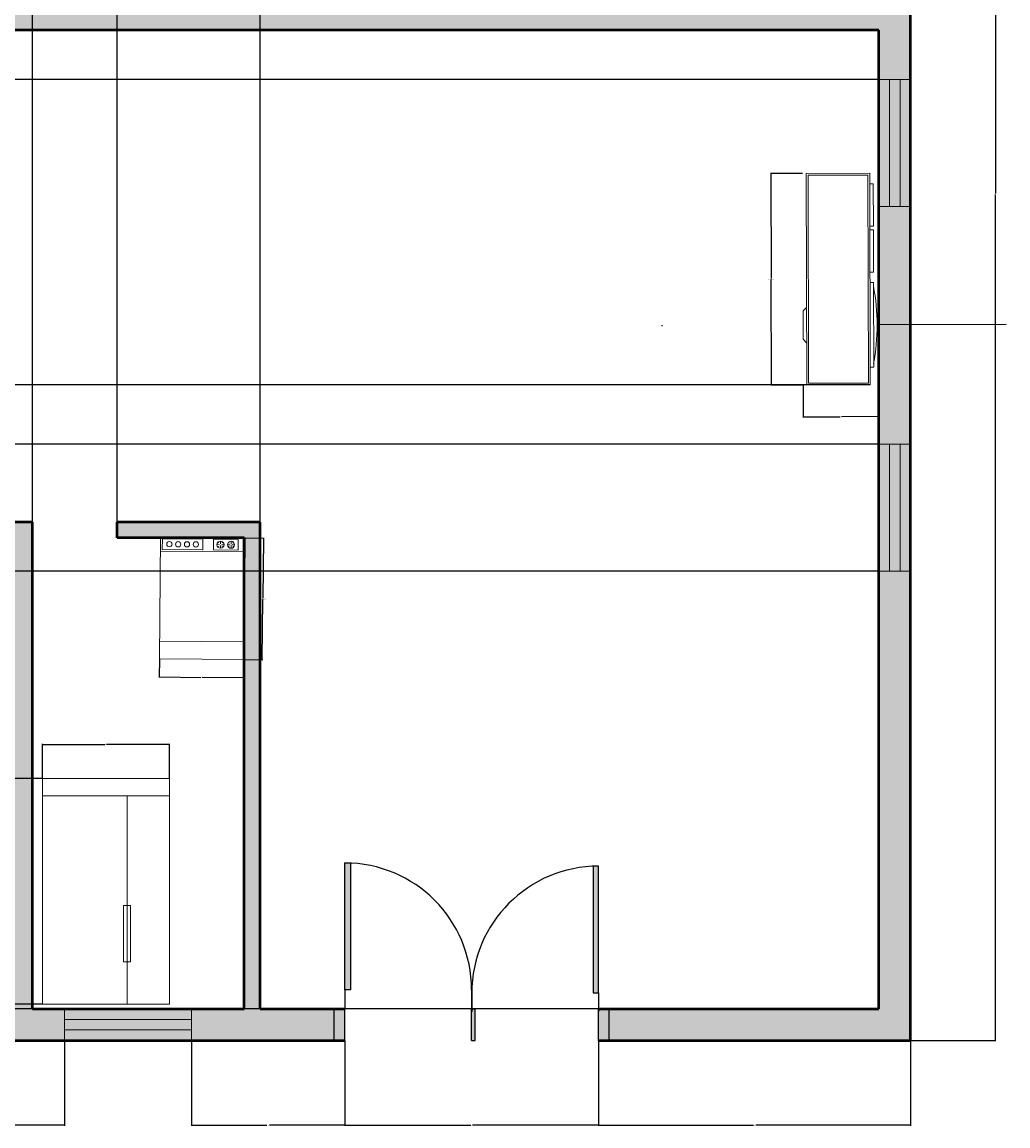
# Model space of a CAD drawing. Units: inches. Extents: x 1201 to 1754, y 247 to 775.
# Tile 9 of 10: x 1475 to 1754, y 247 to 560. Entities that reach past the tile are written whole.
import ezdxf

# ---------------------------------------------------------------- set-up
doc = ezdxf.new("R2010")
doc.units = ezdxf.units.IN
for name, color, linetype, lineweight in [('A-ANNO-DIMS', 2, 'Continuous', 18), ('A-DOOR', 4, 'Continuous', 25), ('A-EQPM', 9, 'Continuous', 20), ('A-FURN', 8, 'Continuous', 18), ('A-GLAZ', 4, 'Continuous', 18), ('A-GLAZ-PATT', 9, 'Continuous', 13), ('A-WALL', 7, 'Continuous', 50), ('A-WALL-PATT', 9, 'Continuous', 13)]:
    doc.layers.add(name, color=color, linetype=linetype, lineweight=lineweight)
doc.layers.add('A-DOOR-PATT', color=29, linetype='Continuous', lineweight=13, true_color=0x4f342a)
doc.styles.get("Standard").update_dxf_attribs({"font": 'arial.ttf'})
doc.dimstyles.get("Standard").update_dxf_attribs({"dimtxt": 0.18, "dimasz": 0.18, "dimexe": 0.18, "dimexo": 0.0625, "dimgap": 0.09, "dimtad": 0, "dimtih": 1, "dimtoh": 1, "dimdec": 4, "dimzin": 0, "dimdsep": 46, "dimtxsty": 'Standard', "dimcen": 0.09, "dimadec": 0, "dimazin": 0, "dimtfac": 1, "dimtdec": 4, "dimtofl": 0, "dimtmove": 0, "dimatfit": 3, "dimfxl": 1, "dimtolj": 1, "dimtzin": 0, "dimarcsym": 0})

# ---------------------------------------------------------------- blocks, each defined once
blk = doc.blocks.new('*U2')
for p, q in [((0, 0), (0, -6)), ((-40, 0), (-40, -6))]:
    blk.add_line(p, q)
blk.add_lwpolyline([(0, 0), (0, 40), (-1.75, 40), (-1.75, 0)], close=True)
blk.add_arc((0, 0), 40, 90, 180)
blk = doc.blocks.new('*U3')
for p, q in [((0, 0), (0, -6)), ((40, 0), (40, -6))]:
    blk.add_line(p, q)
blk.add_lwpolyline([(0, 0), (0, 40), (1.75, 40), (1.75, 0)], close=True)
blk.add_arc((0, 0), 40, 0, 90)
blk = doc.blocks.new('Entertainment Center')
for p, q in [((-4, 0), (-5, -1)), ((4, 0), (-4, 0)), ((5, -1), (4, 0)), ((-17, -19), (-17, -1)), ((-17, -1), (43, -1)), ((-16.5, -18.5), (-16.5, -1.5)), ((-16.5, -1.5), (42.5, -1.5)), ((42.5, -1.5), (42.5, -18.5)), ((43, -1), (43, -19)), ((42.5, -18.5), (-16.5, -18.5)), ((43, -19), (-17, -19)), ((-12, -20), (-12, -19)), ((12, -20), (-12, -20)), ((12, -19), (12, -20)), ((15, -20), (15, -19)), ((27, -20), (15, -20)), ((27, -19), (27, -20)), ((28, -20), (28, -19)), ((40, -20), (28, -20)), ((40, -19), (40, -20))]:
    blk.add_line(p, q)
blk.add_arc((0, 40), 61, 259.6111, 280.3889)
blk = doc.blocks.new('Dishwasher')
for p, q in [((16, 32.5), (16.75, 32.5)), ((16.5, 32), (16.2942, 31.7942)), ((16.3156, 33.1843), (16.5, 33)), ((17, 32.75), (17, 33.5)), ((17, 32.25), (17, 31.5)), ((18, 32.5), (17.25, 32.5)), ((17.5, 33), (17.6938, 33.1938)), ((17.7061, 31.7939), (17.5, 32)), ((19, 32.5), (19.75, 32.5)), ((19.5, 32), (19.2942, 31.7942)), ((19.3156, 33.1843), (19.5, 33)), ((20, 32.75), (20, 33.5)), ((20, 32.25), (20, 31.5)), ((21, 32.5), (20.25, 32.5)), ((20.5, 33), (20.6938, 33.1938)), ((20.7061, 31.7939), (20.5, 32)), ((24, 30.5), (0, 30.5)), ((0, 5), (24, 5))]:
    blk.add_line(p, q)
for points in [[(0, 0), (0, 34.5), (24, 34.5), (24, 0)], [(0.5, 31), (0.5, 34), (12, 34), (12, 31)], [(15, 31), (15, 34), (22, 34), (22, 31)]]:
    blk.add_lwpolyline(points, close=True)
for centre, radius in [((2.5, 32.5), 0.75), ((5, 32.5), 0.75), ((7.5, 32.5), 0.75), ((10, 32.5), 0.75), ((17, 32.5), 1), ((20, 32.5), 1)]:
    blk.add_circle(centre, radius)
blk = doc.blocks.new('Refrigerator-2 door - 36 in front')
for p, q in [((12, 5), (12, 64)), ((0, 5), (36, 5))]:
    blk.add_line(p, q)
for points in [[(0, 0), (0, 64), (36, 64), (36, 0)], [(11, 36), (11, 52), (13, 52), (13, 36)]]:
    blk.add_lwpolyline(points, close=True)
blk = doc.blocks.new('WIN-36IN-PLAN')
for p, q in [((9, 36), (0, 36)), ((3, 0), (3, 36)), ((6, 0), (6, 36))]:
    blk.add_line(p, q)
blk.add_lwpolyline([(0, 36), (0, 0), (9, 0), (9, 36)])
blk = doc.blocks.new('*D33')
at = {"layer": 'A-ANNO-DIMS', "color": 0, "lineweight": -2, "transparency": 16777216}
for p, q in [((1695.85, 516.78), (1686.73, 516.76)), ((1686.91, 516.59), (1686.98, 486.95)), ((1687.05, 456.95), (1686.98, 486.58)), ((1695.98, 456.79), (1686.87, 456.76))]:
    blk.add_line(p, q, dxfattribs=at)
at = {"layer": 'A-ANNO-DIMS', "color": 0, "transparency": 16777216}
for points in [[(1686.94, 516.59), (1686.88, 516.59), (1686.91, 516.77)], [(1687.08, 456.95), (1687.02, 456.95), (1687.05, 456.77)]]:
    blk.add_solid(points, dxfattribs=at)
at = {"layer": 'Defpoints', "color": 0, "transparency": 16777216}
for p in [(1686.91, 516.77), (1695.91, 516.79), (1696.05, 456.79)]:
    blk.add_point(p, dxfattribs=at)
at = {"layer": 'A-ANNO-DIMS', "color": 0, "transparency": 16777216, "insert": (1686.98, 486.77), "char_height": 0.18, "attachment_point": 5}
blk.add_mtext('\\A1;MEDIA UNIT 60', dxfattribs=at)
blk = doc.blocks.new('*D34')
at = {"layer": 'A-ANNO-DIMS', "color": 0, "lineweight": -2, "transparency": 16777216}
for p, q in [((1696.05, 456.72), (1696.07, 447.61)), ((1717.38, 456.77), (1717.4, 447.65)), ((1696.25, 447.79), (1706.53, 447.81)), ((1717.22, 447.83), (1706.94, 447.81))]:
    blk.add_line(p, q, dxfattribs=at)
at = {"layer": 'A-ANNO-DIMS', "color": 0, "transparency": 16777216}
for points in [[(1696.25, 447.82), (1696.25, 447.76), (1696.07, 447.79)], [(1717.22, 447.86), (1717.22, 447.8), (1717.4, 447.83)]]:
    blk.add_solid(points, dxfattribs=at)
at = {"layer": 'Defpoints', "color": 0, "transparency": 16777216}
for p in [(1696.05, 456.79), (1717.38, 456.83), (1696.07, 447.79)]:
    blk.add_point(p, dxfattribs=at)
at = {"layer": 'A-ANNO-DIMS', "color": 0, "transparency": 16777216, "insert": (1706.73, 447.81), "char_height": 0.18, "attachment_point": 5}
blk.add_mtext('\\A1;21', dxfattribs=at)
blk = doc.blocks.new('*D41')
at = {"layer": 'A-ANNO-DIMS', "color": 0, "lineweight": -2, "transparency": 16777216}
for p, q in [((1537.87, 413.46), (1543.17, 413.41)), ((1542.98, 413.23), (1542.82, 396.35)), ((1542.65, 379.09), (1542.81, 395.98)), ((1537.53, 378.96), (1542.83, 378.91))]:
    blk.add_line(p, q, dxfattribs=at)
at = {"layer": 'A-ANNO-DIMS', "color": 0, "transparency": 16777216}
for points in [[(1542.95, 413.23), (1543.01, 413.23), (1542.99, 413.41)], [(1542.62, 379.09), (1542.68, 379.09), (1542.65, 378.91)]]:
    blk.add_solid(points, dxfattribs=at)
at = {"layer": 'Defpoints', "color": 0, "transparency": 16777216}
for p in [(1537.81, 413.46), (1542.99, 413.41), (1537.47, 378.96)]:
    blk.add_point(p, dxfattribs=at)
at = {"layer": 'A-ANNO-DIMS', "color": 0, "transparency": 16777216, "insert": (1542.82, 396.16), "char_height": 0.18, "attachment_point": 5}
blk.add_mtext('\\A1;DISHWASHER 35', dxfattribs=at)
blk = doc.blocks.new('*D42')
at = {"layer": 'A-ANNO-DIMS', "color": 0, "lineweight": -2, "transparency": 16777216}
for p, q in [((1513.47, 379.14), (1513.42, 373.85)), ((1537.47, 378.9), (1537.42, 373.61)), ((1513.6, 374.02), (1525.2, 373.91)), ((1537.24, 373.79), (1525.64, 373.91))]:
    blk.add_line(p, q, dxfattribs=at)
at = {"layer": 'A-ANNO-DIMS', "color": 0, "transparency": 16777216}
for points in [[(1513.6, 374.05), (1513.6, 373.99), (1513.42, 374.03)], [(1537.24, 373.82), (1537.24, 373.76), (1537.42, 373.79)]]:
    blk.add_solid(points, dxfattribs=at)
at = {"layer": 'Defpoints', "color": 0, "transparency": 16777216}
for p in [(1513.47, 379.2), (1537.47, 378.96), (1537.42, 373.79)]:
    blk.add_point(p, dxfattribs=at)
at = {"layer": 'A-ANNO-DIMS', "color": 0, "transparency": 16777216, "insert": (1525.42, 373.91), "char_height": 0.18, "attachment_point": 5}
blk.add_mtext('\\A1;24', dxfattribs=at)
blk = doc.blocks.new('*D43')
at = {"layer": 'A-ANNO-DIMS', "color": 0, "lineweight": -2, "transparency": 16777216}
for p, q in [((1480.23, 345.28), (1470.51, 345.28)), ((1470.69, 345.1), (1470.69, 313.47)), ((1470.69, 281.46), (1470.69, 313.1)), ((1480.23, 281.28), (1470.51, 281.28))]:
    blk.add_line(p, q, dxfattribs=at)
at = {"layer": 'A-ANNO-DIMS', "color": 0, "transparency": 16777216}
for points in [[(1470.66, 345.1), (1470.72, 345.1), (1470.69, 345.28)], [(1470.66, 281.46), (1470.72, 281.46), (1470.69, 281.28)]]:
    blk.add_solid(points, dxfattribs=at)
at = {"layer": 'Defpoints', "color": 0, "transparency": 16777216}
for p in [(1480.29, 345.28), (1470.69, 281.28), (1480.29, 281.28)]:
    blk.add_point(p, dxfattribs=at)
at = {"layer": 'A-ANNO-DIMS', "color": 0, "transparency": 16777216, "insert": (1470.69, 313.28), "char_height": 0.18, "attachment_point": 5}
blk.add_mtext('\\A1;REFRIGERATOR 64', dxfattribs=at)
blk = doc.blocks.new('*D44')
at = {"layer": 'A-ANNO-DIMS', "color": 0, "lineweight": -2, "transparency": 16777216}
for p, q in [((1480.29, 345.35), (1480.29, 355.06)), ((1480.47, 354.88), (1498.07, 354.88)), ((1516.11, 354.88), (1498.51, 354.88)), ((1516.29, 345.35), (1516.29, 355.06))]:
    blk.add_line(p, q, dxfattribs=at)
at = {"layer": 'A-ANNO-DIMS', "color": 0, "transparency": 16777216}
for points in [[(1480.47, 354.91), (1480.47, 354.85), (1480.29, 354.88)], [(1516.11, 354.91), (1516.11, 354.85), (1516.29, 354.88)]]:
    blk.add_solid(points, dxfattribs=at)
at = {"layer": 'Defpoints', "color": 0, "transparency": 16777216}
for p in [(1480.29, 354.88), (1480.29, 345.28), (1516.29, 345.28)]:
    blk.add_point(p, dxfattribs=at)
at = {"layer": 'A-ANNO-DIMS', "color": 0, "transparency": 16777216, "insert": (1498.29, 354.88), "char_height": 0.18, "attachment_point": 5}
blk.add_mtext('\\A1;36', dxfattribs=at)
blk = doc.blocks.new('*D46')
at = {"layer": 'A-ANNO-DIMS', "color": 0, "lineweight": -2, "transparency": 16777216}
for p, q in [((1726.58, 750.94), (1750.72, 750.94)), ((1750.54, 750.76), (1750.54, 511.12)), ((1750.54, 271.12), (1750.54, 510.76)), ((1726.58, 270.94), (1750.72, 270.94))]:
    blk.add_line(p, q, dxfattribs=at)
at = {"layer": 'A-ANNO-DIMS', "color": 0, "transparency": 16777216}
for points in [[(1750.51, 750.76), (1750.57, 750.76), (1750.54, 750.94)], [(1750.51, 271.12), (1750.57, 271.12), (1750.54, 270.94)]]:
    blk.add_solid(points, dxfattribs=at)
at = {"layer": 'Defpoints', "color": 0, "transparency": 16777216}
for p in [(1726.52, 750.94), (1750.54, 750.94), (1726.52, 270.94)]:
    blk.add_point(p, dxfattribs=at)
at = {"layer": 'A-ANNO-DIMS', "color": 0, "transparency": 16777216, "insert": (1750.54, 510.94), "char_height": 0.18, "attachment_point": 5}
blk.add_mtext('\\A1;480', dxfattribs=at)
blk = doc.blocks.new('*D55')
at = {"layer": 'A-ANNO-DIMS', "color": 0, "lineweight": -2, "transparency": 16777216}
for p, q in [((1501.52, 418), (1501.52, 775.14)), ((1501.7, 774.96), (1521.44, 774.96)), ((1541.84, 774.96), (1522.1, 774.96)), ((1542.02, 418), (1542.02, 775.14))]:
    blk.add_line(p, q, dxfattribs=at)
at = {"layer": 'A-ANNO-DIMS', "color": 0, "transparency": 16777216}
for points in [[(1501.7, 774.99), (1501.7, 774.93), (1501.52, 774.96)], [(1541.84, 774.99), (1541.84, 774.93), (1542.02, 774.96)]]:
    blk.add_solid(points, dxfattribs=at)
at = {"layer": 'Defpoints', "color": 0, "transparency": 16777216}
for p in [(1542.02, 774.96), (1501.52, 417.94), (1542.02, 417.94)]:
    blk.add_point(p, dxfattribs=at)
at = {"layer": 'A-ANNO-DIMS', "color": 0, "transparency": 16777216, "insert": (1521.77, 774.96), "char_height": 0.18, "attachment_point": 5}
blk.add_mtext('\\A1;40.5', dxfattribs=at)
blk = doc.blocks.new('*D56')
at = {"layer": 'A-ANNO-DIMS', "color": 0, "lineweight": -2, "transparency": 16777216}
for p, q in [((1566.02, 270.88), (1566.02, 246.75)), ((1638.02, 270.88), (1638.02, 246.75)), ((1566.2, 246.93), (1601.8, 246.93)), ((1637.84, 246.93), (1602.24, 246.93))]:
    blk.add_line(p, q, dxfattribs=at)
at = {"layer": 'A-ANNO-DIMS', "color": 0, "transparency": 16777216}
for points in [[(1566.2, 246.96), (1566.2, 246.9), (1566.02, 246.93)], [(1637.84, 246.96), (1637.84, 246.9), (1638.02, 246.93)]]:
    blk.add_solid(points, dxfattribs=at)
at = {"layer": 'Defpoints', "color": 0, "transparency": 16777216}
for p in [(1566.02, 270.94), (1638.02, 270.94), (1638.02, 246.93)]:
    blk.add_point(p, dxfattribs=at)
at = {"layer": 'A-ANNO-DIMS', "color": 0, "transparency": 16777216, "insert": (1602.02, 246.93), "char_height": 0.18, "attachment_point": 5}
blk.add_mtext('\\A1;72', dxfattribs=at)
blk = doc.blocks.new('*D57')
at = {"layer": 'A-ANNO-DIMS', "color": 0, "lineweight": -2, "transparency": 16777216}
for p, q in [((1638.02, 270.88), (1638.02, 246.75)), ((1726.52, 270.88), (1726.52, 246.75)), ((1638.2, 246.93), (1681.95, 246.93)), ((1726.34, 246.93), (1682.6, 246.93))]:
    blk.add_line(p, q, dxfattribs=at)
at = {"layer": 'A-ANNO-DIMS', "color": 0, "transparency": 16777216}
for points in [[(1638.2, 246.96), (1638.2, 246.9), (1638.02, 246.93)], [(1726.34, 246.96), (1726.34, 246.9), (1726.52, 246.93)]]:
    blk.add_solid(points, dxfattribs=at)
at = {"layer": 'Defpoints', "color": 0, "transparency": 16777216}
for p in [(1638.02, 270.94), (1726.52, 270.94), (1726.52, 246.93)]:
    blk.add_point(p, dxfattribs=at)
at = {"layer": 'A-ANNO-DIMS', "color": 0, "transparency": 16777216, "insert": (1682.27, 246.93), "char_height": 0.18, "attachment_point": 5}
blk.add_mtext('\\A1;88.5', dxfattribs=at)
blk = doc.blocks.new('*D60')
at = {"layer": 'A-ANNO-DIMS', "color": 0, "lineweight": -2, "transparency": 16777216}
for p, q in [((1477.52, 418), (1477.52, 775.14)), ((1477.7, 774.96), (1489.3, 774.96)), ((1501.34, 774.96), (1489.74, 774.96)), ((1501.52, 418), (1501.52, 775.14))]:
    blk.add_line(p, q, dxfattribs=at)
at = {"layer": 'A-ANNO-DIMS', "color": 0, "transparency": 16777216}
for points in [[(1477.7, 774.99), (1477.7, 774.93), (1477.52, 774.96)], [(1501.34, 774.99), (1501.34, 774.93), (1501.52, 774.96)]]:
    blk.add_solid(points, dxfattribs=at)
at = {"layer": 'Defpoints', "color": 0, "transparency": 16777216}
for p in [(1501.52, 774.96), (1477.52, 417.94), (1501.52, 417.94)]:
    blk.add_point(p, dxfattribs=at)
at = {"layer": 'A-ANNO-DIMS', "color": 0, "transparency": 16777216, "insert": (1489.52, 774.96), "char_height": 0.18, "attachment_point": 5}
blk.add_mtext('\\A1;24', dxfattribs=at)
blk = doc.blocks.new('*D74')
at = {"layer": 'A-ANNO-DIMS', "color": 0, "lineweight": -2, "transparency": 16777216}
for p, q in [((1717.46, 404.03), (1222.33, 404.03)), ((1222.51, 403.85), (1222.51, 342.17)), ((1222.51, 280.12), (1222.51, 341.81)), ((1717.46, 279.94), (1222.33, 279.94))]:
    blk.add_line(p, q, dxfattribs=at)
at = {"layer": 'A-ANNO-DIMS', "color": 0, "transparency": 16777216}
for points in [[(1222.48, 403.85), (1222.54, 403.85), (1222.51, 404.03)], [(1222.48, 280.12), (1222.54, 280.12), (1222.51, 279.94)]]:
    blk.add_solid(points, dxfattribs=at)
at = {"layer": 'Defpoints', "color": 0, "transparency": 16777216}
for p in [(1222.51, 404.03), (1717.52, 404.03), (1717.52, 279.94)]:
    blk.add_point(p, dxfattribs=at)
at = {"layer": 'A-ANNO-DIMS', "color": 0, "transparency": 16777216, "insert": (1222.51, 341.99), "char_height": 0.18, "attachment_point": 5}
blk.add_mtext('\\A1;124.1', dxfattribs=at)
blk = doc.blocks.new('*D75')
at = {"layer": 'A-ANNO-DIMS', "color": 0, "lineweight": -2, "transparency": 16777216}
for p, q in [((1717.46, 557.44), (1222.33, 557.44)), ((1222.51, 557.26), (1222.51, 550.62)), ((1222.51, 543.62), (1222.51, 550.26)), ((1717.46, 543.44), (1222.33, 543.44))]:
    blk.add_line(p, q, dxfattribs=at)
at = {"layer": 'A-ANNO-DIMS', "color": 0, "transparency": 16777216}
for points in [[(1222.48, 557.26), (1222.54, 557.26), (1222.51, 557.44)], [(1222.48, 543.62), (1222.54, 543.62), (1222.51, 543.44)]]:
    blk.add_solid(points, dxfattribs=at)
at = {"layer": 'Defpoints', "color": 0, "transparency": 16777216}
for p in [(1222.51, 557.44), (1717.52, 557.44), (1717.52, 543.44)]:
    blk.add_point(p, dxfattribs=at)
at = {"layer": 'A-ANNO-DIMS', "color": 0, "transparency": 16777216, "insert": (1222.51, 550.44), "char_height": 0.18, "attachment_point": 5}
blk.add_mtext('\\A1;14.005', dxfattribs=at)
blk = doc.blocks.new('*D79')
at = {"layer": 'A-ANNO-DIMS', "color": 0, "lineweight": -2, "transparency": 16777216}
for p, q in [((1399.01, 270.88), (1399.01, 246.75)), ((1486.59, 270.88), (1486.59, 246.75)), ((1399.19, 246.93), (1442.41, 246.93)), ((1486.41, 246.93), (1443.19, 246.93))]:
    blk.add_line(p, q, dxfattribs=at)
at = {"layer": 'A-ANNO-DIMS', "color": 0, "transparency": 16777216}
for points in [[(1399.19, 246.96), (1399.19, 246.9), (1399.01, 246.93)], [(1486.41, 246.96), (1486.41, 246.9), (1486.59, 246.93)]]:
    blk.add_solid(points, dxfattribs=at)
at = {"layer": 'Defpoints', "color": 0, "transparency": 16777216}
for p in [(1399.01, 270.94), (1486.59, 270.94), (1486.59, 246.93)]:
    blk.add_point(p, dxfattribs=at)
at = {"layer": 'A-ANNO-DIMS', "color": 0, "transparency": 16777216, "insert": (1442.8, 246.93), "char_height": 0.18, "attachment_point": 5}
blk.add_mtext('\\A1;87.58', dxfattribs=at)
blk = doc.blocks.new('*D80')
at = {"layer": 'A-ANNO-DIMS', "color": 0, "lineweight": -2, "transparency": 16777216}
for p, q in [((1522.59, 270.88), (1522.59, 246.75)), ((1566.02, 270.88), (1566.02, 246.75)), ((1522.77, 246.93), (1543.91, 246.93)), ((1565.84, 246.93), (1544.7, 246.93))]:
    blk.add_line(p, q, dxfattribs=at)
at = {"layer": 'A-ANNO-DIMS', "color": 0, "transparency": 16777216}
for points in [[(1522.77, 246.96), (1522.77, 246.9), (1522.59, 246.93)], [(1565.84, 246.96), (1565.84, 246.9), (1566.02, 246.93)]]:
    blk.add_solid(points, dxfattribs=at)
at = {"layer": 'Defpoints', "color": 0, "transparency": 16777216}
for p in [(1522.59, 270.94), (1566.02, 270.94), (1566.02, 246.93)]:
    blk.add_point(p, dxfattribs=at)
at = {"layer": 'A-ANNO-DIMS', "color": 0, "transparency": 16777216, "insert": (1544.31, 246.93), "char_height": 0.18, "attachment_point": 5}
blk.add_mtext('\\A1;43.43', dxfattribs=at)
blk = doc.blocks.new('*D96')
at = {"layer": 'A-ANNO-DIMS', "color": 0, "lineweight": -2, "transparency": 16777216}
for p, q in [((1714.98, 456.83), (1222.33, 456.83)), ((1222.51, 456.65), (1222.51, 448.61)), ((1222.51, 440.21), (1222.51, 448.25)), ((1717.46, 440.03), (1222.33, 440.03))]:
    blk.add_line(p, q, dxfattribs=at)
at = {"layer": 'A-ANNO-DIMS', "color": 0, "transparency": 16777216}
for points in [[(1222.48, 456.65), (1222.54, 456.65), (1222.51, 456.83)], [(1222.48, 440.21), (1222.54, 440.21), (1222.51, 440.03)]]:
    blk.add_solid(points, dxfattribs=at)
at = {"layer": 'Defpoints', "color": 0, "transparency": 16777216}
for p in [(1222.51, 456.83), (1715.05, 456.83), (1717.52, 440.03)]:
    blk.add_point(p, dxfattribs=at)
at = {"layer": 'A-ANNO-DIMS', "color": 0, "transparency": 16777216, "insert": (1222.51, 448.43), "char_height": 0.18, "attachment_point": 5}
blk.add_mtext('\\A1;16.793', dxfattribs=at)
blk = doc.blocks.new('*D102')
at = {"layer": 'A-ANNO-DIMS', "color": 0, "lineweight": -2, "transparency": 16777216}
for p, q in [((1655.92, 473.7), (1656.1, 473.7)), ((1656.01, 473.61), (1656.01, 473.79)), ((1753.61, 473.91), (1717.19, 473.83))]:
    blk.add_line(p, q, dxfattribs=at)
at = {"layer": 'A-ANNO-DIMS', "color": 0, "transparency": 16777216}
blk.add_solid([(1717.19, 473.86), (1717.19, 473.8), (1717.01, 473.83)], dxfattribs=at)
at = {"layer": 'Defpoints', "color": 0, "transparency": 16777216}
for p in [(1656.01, 473.7), (1717.01, 473.83)]:
    blk.add_point(p, dxfattribs=at)
at = {"layer": 'A-ANNO-DIMS', "color": 0, "transparency": 16777216, "insert": (1753.9, 473.91), "char_height": 0.18, "attachment_point": 5}
blk.add_mtext('\\A1;R61', dxfattribs=at)

msp = doc.modelspace()

# ---------------------------------------------------------------- hatches: boundary and pattern name
at = {"layer": 'A-DOOR-PATT'}
h = msp.add_hatch(color=256, dxfattribs=at)
h.dxf.hatch_style = 1
h.paths.add_polyline_path([(1391.9756, 612.6194), (1390.4026, 612.6194), (1390.4026, 576.699, 0.01094143), (1391.9756, 576.6646)])
h.paths.add_polyline_path([(1471.5208, 621.9415), (1459.5208, 621.9415), (1459.5208, 617.4415), (1471.5208, 617.4415)])
h.paths.add_polyline_path([(1459.4756, 663.2896, 0.01094143), (1457.9026, 663.2551), (1457.9026, 627.3347), (1459.4756, 627.3347)])
h.paths.add_polyline_path([(1477.5208, 602.9415), (1471.5208, 602.9415), (1471.5208, 599.9415), (1477.5208, 599.9415)])
h.paths.add_polyline_path([(1518.8344, 565.5145), (1482.914, 565.5145), (1482.914, 563.9415), (1518.8689, 563.9415, 0.01094143)])
h.paths.add_polyline_path([(1477.5208, 563.9415), (1471.5208, 563.9415), (1471.5208, 561.9692), (1477.5208, 561.9692)])
h.paths.add_polyline_path([(1621.5208, 674.4415), (1618.5208, 674.4415), (1618.5208, 669.9415), (1621.5208, 669.9415)])
h.paths.add_polyline_path([(1660.5208, 674.4415), (1657.5208, 674.4415), (1657.5208, 669.9415), (1660.5208, 669.9415)])
h.paths.add_polyline_path([(1657.509, 715.7896, 0.01094143), (1655.936, 715.7551), (1655.936, 679.8347), (1657.509, 679.8347)])
h.paths.add_polyline_path([(1566.0208, 279.9415), (1563.0208, 279.9415), (1563.0208, 270.9415), (1566.0208, 270.9415)])
h.paths.add_polyline_path([(1567.6389, 321.2551, 0.01094143), (1566.0659, 321.2896), (1566.0659, 285.3347), (1567.6389, 285.3347)])
h.paths.add_polyline_path([(1603.0208, 279.9415), (1602.0208, 279.9415), (1602.0208, 270.9415), (1603.0208, 270.9415)])
h.paths.add_polyline_path([(1641.0208, 279.9415), (1638.0208, 279.9415), (1638.0208, 270.9415), (1641.0208, 270.9415)])
h.paths.add_polyline_path([(1638.0208, 320.3922, 0.01094143), (1636.4477, 320.3578), (1636.4477, 284.4374), (1638.0208, 284.4374)])
at = {"layer": 'A-GLAZ-PATT'}
h = msp.add_hatch(color=256, dxfattribs=at)
h.dxf.hatch_style = 1
h.set_gradient(color1=(0, 0, 255), color2=(255, 255, 0), name='INVHEMISPHERICAL')
h.paths.add_polyline_path([(1720.5208, 543.4363), (1717.5208, 543.4363), (1717.5208, 507.4363), (1720.5208, 507.4363)])
h.paths.add_polyline_path([(1723.5208, 543.4363), (1720.5208, 543.4363), (1720.5208, 507.4363), (1723.5208, 507.4363)])
h.paths.add_polyline_path([(1726.5208, 543.4363), (1723.5208, 543.4363), (1723.5208, 507.4363), (1726.5208, 507.4363)])
h = msp.add_hatch(color=256, dxfattribs=at)
h.dxf.hatch_style = 1
h.set_gradient(color1=(0, 0, 255), color2=(255, 255, 0), name='INVCURVED')
h.paths.add_polyline_path([(1726.5208, 440.0342), (1723.5208, 440.0342), (1723.5208, 404.0342), (1726.5208, 404.0342)])
h.paths.add_polyline_path([(1723.5208, 440.0342), (1720.5208, 440.0342), (1720.5208, 404.0342), (1723.5208, 404.0342)])
h.paths.add_polyline_path([(1720.5208, 440.0342), (1717.5208, 440.0342), (1717.5208, 404.0342), (1720.5208, 404.0342)])
h = msp.add_hatch(color=256, dxfattribs=at)
h.dxf.hatch_style = 1
h.set_gradient(color1=(0, 0, 255), color2=(255, 255, 0), name='INVCURVED')
h.paths.add_polyline_path([(1522.5907, 279.9415), (1486.5907, 279.9415), (1486.5907, 276.9415), (1522.5907, 276.9415)])
h.paths.add_polyline_path([(1522.5907, 276.9415), (1486.5907, 276.9415), (1486.5907, 273.9415), (1522.5907, 273.9415)])
h.paths.add_polyline_path([(1522.5907, 273.9415), (1486.5907, 273.9415), (1486.5907, 270.9415), (1522.5907, 270.9415)])
at = {"layer": 'A-WALL-PATT'}
h = msp.add_hatch(color=256, dxfattribs=at)
h.dxf.hatch_style = 1
h.paths.add_polyline_path([(1255.5208, 741.9415), (1471.5208, 741.9415), (1471.5208, 684.2327), (1471.5208, 602.9415), (1477.5208, 602.9415), (1477.5208, 669.9415), (1618.5208, 669.9415), (1618.5208, 674.4415), (1477.5208, 674.4415), (1477.5208, 741.9415), (1481.2969, 741.9415), (1481.2969, 750.9415), (1246.5208, 750.9415), (1246.5208, 700.7954), (1255.5208, 700.7954)])
h.paths.add_polyline_path([(1255.5208, 557.4415), (1399.5208, 557.4415), (1399.5208, 617.4415), (1423.5208, 617.4415), (1423.5208, 621.9415), (1392.0208, 621.9415), (1392.0208, 617.4415), (1395.0208, 617.4415), (1395.0208, 561.9415), (1255.5208, 561.9415), (1255.5208, 571.8878), (1246.5208, 571.8878), (1246.5208, 506.6967), (1255.5208, 506.6967)])
h.paths.add_polyline_path([(1255.5208, 664.7954), (1246.5208, 664.7954), (1246.5208, 595.8878), (1255.398, 595.8878), (1255.398, 617.4415), (1315.398, 617.4415), (1356.0208, 617.4415), (1356.0208, 618.0127), (1356.0208, 621.9415), (1255.5208, 621.9415), (1255.5208, 629.6628)])
h.paths.add_polyline_path([(1255.5208, 470.6967), (1246.5208, 470.6967), (1246.5208, 347.7487), (1255.5208, 347.7487), (1255.5208, 413.4415), (1405.5208, 413.4415), (1405.5208, 417.9415), (1255.5208, 417.9415)])
h.paths.add_polyline_path([(1290.9481, 279.9415), (1255.5208, 279.9415), (1255.5208, 311.7487), (1246.5208, 311.7487), (1246.5208, 270.9415), (1290.9481, 270.9415)])
h.paths.add_polyline_path([(1486.5907, 279.9415), (1477.5208, 279.9415), (1477.5208, 417.9415), (1468.5208, 417.9415), (1468.5208, 413.4415), (1471.5208, 413.4415), (1471.5208, 279.9415), (1399.0105, 279.9415), (1399.0105, 270.9415), (1486.5907, 270.9415)])
h.paths.add_polyline_path([(1563.0208, 279.9415), (1542.0208, 279.9415), (1542.0208, 417.9415), (1501.5208, 417.9415), (1501.5208, 413.4415), (1513.81, 413.4415), (1513.8125, 413.6987), (1537.8114, 413.4623), (1537.5208, 383.9637), (1537.5208, 279.9415), (1522.5907, 279.9415), (1522.5907, 270.9415), (1563.0208, 270.9415)])
h.paths.add_polyline_path([(1726.5208, 404.0342), (1717.5208, 404.0342), (1717.5208, 279.9415), (1641.0208, 279.9415), (1641.0208, 270.9415), (1726.5208, 270.9415)])
h.paths.add_polyline_path([(1726.5208, 507.4363), (1717.5208, 507.4363), (1717.5208, 440.0342), (1726.5208, 440.0342)])
h.paths.add_polyline_path([(1726.5208, 611.6009), (1717.5208, 611.6009), (1717.5208, 561.9415), (1477.5208, 561.9415), (1471.5208, 561.9692), (1471.5208, 557.4415), (1717.5208, 557.4415), (1717.5208, 543.4363), (1726.5208, 543.4363)])
h.paths.add_polyline_path([(1726.5208, 750.9415), (1505.2969, 750.9415), (1505.2969, 741.9415), (1697.6884, 741.9415), (1697.6884, 741.9922), (1718.6884, 741.9922), (1718.6884, 733.9922), (1717.5208, 733.9922), (1717.5208, 674.4415), (1660.5208, 674.4415), (1660.5208, 669.9415), (1717.5208, 669.9415), (1717.5208, 647.6009), (1726.5208, 647.6009)])

# ---------------------------------------------------------------- linework, layer by layer
at = {"layer": 'A-DOOR'}
for p, q in [((1563.0208, 270.9415), (1563.0208, 279.9415)), ((1566.0208, 270.9415), (1566.0208, 279.9415)), ((1602.0208, 270.9415), (1602.0208, 279.9415)), ((1602.0208, 279.9415), (1603.0208, 279.9415)), ((1603.0208, 270.9415), (1603.0208, 279.9415)), ((1638.0208, 270.9415), (1638.0208, 279.9415)), ((1641.0208, 270.9415), (1641.0208, 279.9415)), ((1602.0208, 270.9415), (1603.0208, 270.9415))]:
    msp.add_line(p, q, dxfattribs=at)
at = {"layer": 'A-WALL'}
for p, q in [((1717.5208, 557.4415), (1471.5208, 557.4415)), ((1717.5208, 279.9415), (1717.5208, 557.4415)), ((1477.5208, 417.9415), (1468.5208, 417.9415)), ((1477.5208, 279.9415), (1477.5208, 417.9415)), ((1542.0208, 417.9415), (1501.5208, 417.9415)), ((1501.5208, 413.4415), (1501.5208, 417.9415)), ((1542.0208, 279.9415), (1542.0208, 417.9415)), ((1537.5208, 413.4415), (1501.5208, 413.4415)), ((1537.5208, 279.9415), (1537.5208, 413.4415)), ((1477.5208, 279.9415), (1537.5208, 279.9415)), ((1542.0208, 279.9415), (1566.0208, 279.9415)), ((1638.0208, 279.9415), (1717.5208, 279.9415))]:
    msp.add_line(p, q, dxfattribs=at)
msp.add_lwpolyline([(1638.0208, 270.9415), (1726.5208, 270.9415), (1726.5208, 750.9415), (1246.5208, 750.9415), (1246.5208, 270.9415), (1566.0208, 270.9415)], dxfattribs=at)

# ---------------------------------------------------------------- block references
at = {"layer": 'A-DOOR', "xscale": 0.8988714898198789, "yscale": 0.8988714898198789, "zscale": 0.8988714898198789}
for name, p in [('*U3', (1566.0659, 285.3347)), ('*U3', (1566.0659, 285.3347)), ('*U2', (1638.0208, 284.4374))]:
    msp.add_blockref(name, p, dxfattribs=at)
at = {"layer": 'A-EQPM'}
for name, p, rotation in [('Dishwasher', (1513.4727, 379.2004), 359.4355542195772), ('Refrigerator-2 door - 36 in front', (1516.2925, 345.284), 180)]:
    msp.add_blockref(name, p, dxfattribs=dict(at, rotation=rotation))
at = {"layer": 'A-FURN', "rotation": 90.12679107421874}
msp.add_blockref('Entertainment Center', (1696.0093, 473.7852), dxfattribs=at)
at = {"layer": 'A-GLAZ'}
for p in [(1717.5208, 507.4363), (1717.5208, 404.0342)]:
    msp.add_blockref('WIN-36IN-PLAN', p, dxfattribs=at)
at = {"layer": 'A-GLAZ', "rotation": 90.00000000000115}
msp.add_blockref('WIN-36IN-PLAN', (1522.5907, 270.9415), dxfattribs=at)

# ---------------------------------------------------------------- dimensions: what is measured, and where the dimension line sits
at = {"layer": 'A-ANNO-DIMS'}
for base, p1, p2, override, picture, middle in [((1501.5208, 774.9565), (1477.5208, 417.9415), (1501.5208, 417.9415), {"dimdec": 0, "dimlfac": 1, "dimrnd": 0, "dimzin": 0, "dimdsep": 46, "dimlunit": 2}, '*D60', (1489.5208, 774.9565)), ((1542.0208, 774.9565), (1501.5208, 417.9415), (1542.0208, 417.9415), {"dimdec": 1, "dimlfac": 1, "dimrnd": 0, "dimzin": 0, "dimdsep": 46, "dimlunit": 2}, '*D55', (1521.7708, 774.9565)), ((1486.5907, 246.9265), (1399.0105, 270.9415), (1486.5907, 270.9415), {"dimdec": 2, "dimlfac": 1, "dimrnd": 0, "dimzin": 0, "dimdsep": 46, "dimlunit": 2}, '*D79', (1442.8006, 246.9265)), ((1566.0208, 246.9265), (1522.5907, 270.9415), (1566.0208, 270.9415), {"dimdec": 2, "dimlfac": 1, "dimrnd": 0, "dimzin": 0, "dimdsep": 46, "dimlunit": 2}, '*D80', (1544.3057, 246.9265)), ((1638.0208, 246.9265), (1566.0208, 270.9415), (1638.0208, 270.9415), {"dimdec": 0, "dimlfac": 1, "dimrnd": 0, "dimzin": 0, "dimdsep": 46, "dimlunit": 2}, '*D56', (1602.0208, 246.9265)), ((1726.5208, 246.9265), (1638.0208, 270.9415), (1726.5208, 270.9415), {"dimdec": 1, "dimlfac": 1, "dimrnd": 0, "dimzin": 0, "dimdsep": 46, "dimlunit": 2}, '*D57', (1682.2708, 246.9265))]:
    dim = msp.add_linear_dim(base=base, p1=p1, p2=p2, dimstyle='Standard', override=override, dxfattribs=at)
    dim.commit()
    dim.dimension.update_dxf_attribs({"geometry": picture, "text_midpoint": middle})
for base, p1, p2, angle, override, picture, middle in [((1750.5358, 750.9415), (1726.5208, 270.9415), (1726.5208, 750.9415), 90, {"dimdec": 0, "dimlfac": 1, "dimrnd": 0, "dimzin": 0, "dimdsep": 46, "dimlunit": 2}, '*D46', (1750.5358, 510.9415)), ((1222.5058, 557.4415), (1717.5208, 543.4363), (1717.5208, 557.4415), 90, {"dimdec": 3, "dimlfac": 1, "dimrnd": 0, "dimzin": 0, "dimdsep": 46, "dimlunit": 2}, '*D75', (1222.5058, 550.4389)), ((1222.5058, 456.8273), (1717.5208, 440.0342), (1715.0469, 456.8273), 90, {"dimdec": 3, "dimlfac": 1, "dimrnd": 0, "dimzin": 0, "dimdsep": 46, "dimlunit": 2}, '*D96', (1222.5058, 448.4308)), ((1696.0669, 447.7853), (1717.3802, 456.8325), (1696.047, 456.7853), 180.126791, {"dimdec": 0, "dimlfac": 1, "dimrnd": 0, "dimzin": 0, "dimdsep": 46, "dimlunit": 2}, '*D34', (1706.7335, 447.8089)), ((1222.5058, 404.0342), (1717.5208, 279.9415), (1717.5208, 404.0342), 90, {"dimdec": 1, "dimlfac": 1, "dimrnd": 0, "dimzin": 0, "dimdsep": 46, "dimlunit": 2}, '*D74', (1222.5058, 341.9878)), ((1537.4205, 373.7892), (1513.4727, 379.2004), (1537.4715, 378.9639), 359.435554, {"dimdec": 0, "dimlfac": 1, "dimrnd": 0, "dimzin": 0, "dimdsep": 46, "dimlunit": 2}, '*D42', (1525.4211, 373.9074)), ((1480.2925, 354.884), (1516.2925, 345.284), (1480.2925, 345.284), 180, {"dimdec": 0, "dimlfac": 1, "dimrnd": 0, "dimzin": 0, "dimdsep": 46, "dimlunit": 2}, '*D44', (1498.2925, 354.884))]:
    dim = msp.add_linear_dim(base=base, p1=p1, p2=p2, angle=angle, dimstyle='Standard', override=override, dxfattribs=at)
    dim.commit()
    dim.dimension.update_dxf_attribs({"geometry": picture, "text_midpoint": middle})
for base, p1, p2, angle, text, picture, middle in [((1686.9142, 516.7652), (1696.047, 456.7853), (1695.9142, 516.7851), 90.126791, 'MEDIA UNIT <>', '*D33', (1686.9806, 486.7653)), ((1542.98613, 413.41127), (1537.47151, 378.96393), (1537.81138, 413.46225), 89.435554, 'DISHWASHER <>', '*D41', (1542.81619, 396.16211)), ((1470.6925, 281.284), (1480.2925, 345.284), (1480.2925, 281.284), 270, 'REFRIGERATOR <>', '*D43', (1470.6925, 313.284))]:
    dim = msp.add_linear_dim(base=base, p1=p1, p2=p2, angle=angle, text=text, dimstyle='Standard', override={"dimdec": 0, "dimlfac": 1, "dimrnd": 0, "dimzin": 0, "dimdsep": 46, "dimlunit": 2}, dxfattribs=at)
    dim.commit()
    dim.dimension.update_dxf_attribs({"geometry": picture, "text_midpoint": middle})
dim = msp.add_radius_dim(center=(1656.0094, 473.6967), mpoint=(1717.0093, 473.832), dimstyle='Standard', override={"dimdec": 0, "dimlfac": 1, "dimrnd": 0, "dimzin": 0, "dimdsep": 46, "dimlunit": 2}, dxfattribs=at)
dim.commit()
dim.dimension.update_dxf_attribs({"geometry": '*D102', "text_midpoint": (1753.6092, 473.9132), "dimtype": 164})

doc.saveas('drawing.dxf')
